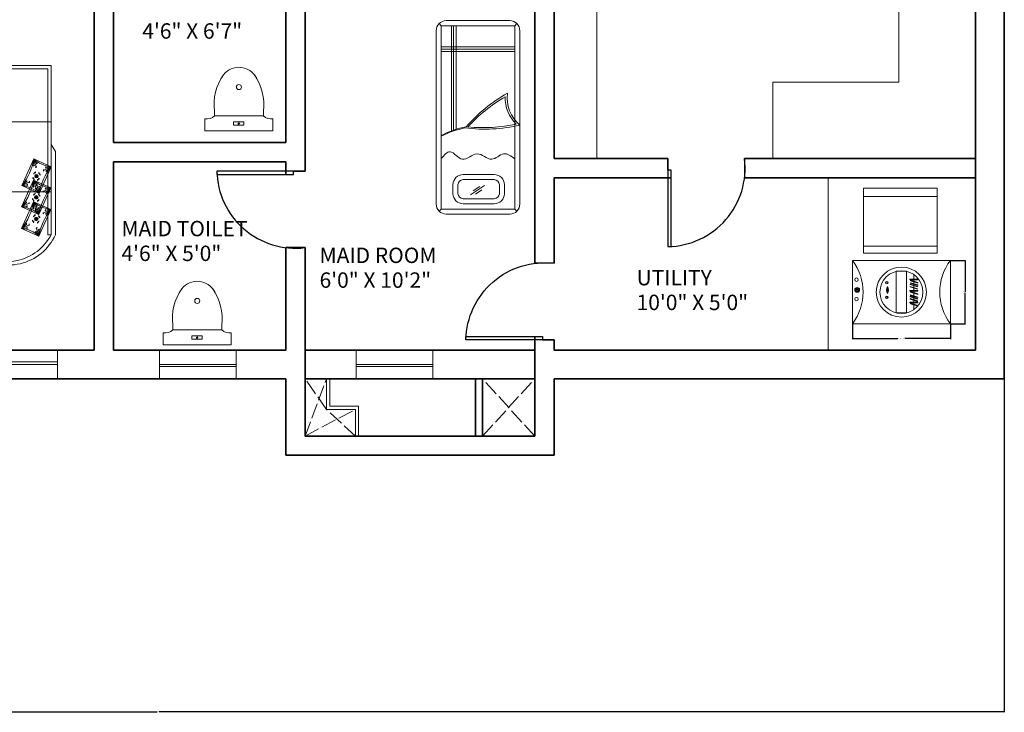
# Model space of a CAD drawing. Units: inches. Extents: x -61 to 1599, y -1316 to 257.
# Tile 167 of 204: x 1214 to 1523, y -1316 to -1099. Entities that reach past the tile are written whole.
import ezdxf

# ---------------------------------------------------------------- set-up
doc = ezdxf.new("R2010")
doc.units = ezdxf.units.IN
doc.header["$MEASUREMENT"] = 0
doc.linetypes.add('ACAD_ISO02W100', pattern=[15, 12, -3])
for name, color, linetype, lineweight in [('A-ANNO-DIMS', 2, 'Continuous', 18), ('A-AREA-IDEN', 1, 'Continuous', 18), ('A-EQPM', 9, 'Continuous', 18), ('A-FLOR-CASE', 8, 'Continuous', 18), ('A-FLOR-FIXT', 8, 'Continuous', 18), ('A-FLOR-OPEN-HIDN', 8, 'ACAD_ISO02W100', 13), ('A-WALL-JAMB', 4, 'ACAD_ISO02W100', 25), ('DOORS', 2, 'Continuous', 25), ('FURNITURE', 83, 'Continuous', 18), ('WALLS', 4, 'Continuous', 35), ('WINDOWS', 220, 'Continuous', 18)]:
    doc.layers.add(name, color=color, linetype=linetype, lineweight=lineweight)
doc.styles.get("Standard").update_dxf_attribs({"font": 'arial.ttf'})
doc.dimstyles.get("Standard").update_dxf_attribs({"dimtxt": 0.18, "dimasz": 0.18, "dimexe": 0.18, "dimexo": 0.0625, "dimgap": 0.09, "dimtad": 0, "dimtih": 1, "dimtoh": 1, "dimdec": 0, "dimzin": 0, "dimdsep": 46, "dimlunit": 3, "dimtxsty": 'Standard', "dimcen": 0.09, "dimadec": 0, "dimazin": 0, "dimtfac": 1, "dimtdec": 0, "dimtofl": 0, "dimtmove": 0, "dimatfit": 3, "dimfxl": 1, "dimtolj": 1, "dimtzin": 0, "dimarcsym": 0})

# ---------------------------------------------------------------- blocks, each defined once
blk = doc.blocks.new('DOOR-SWING-24')
blk.add_line((0, 0), (0, 3.6))
blk.add_lwpolyline([(0, 0), (0, -24), (1.05, -24), (1.05, 0)], close=True)
blk.add_arc((-0.44, 0.62), 24.62, 271.0259, 6.9559)
blk = doc.blocks.new('WIN-24IN')
for p, q in [((0, 4.5), (0, 9)), ((0, 9), (0, 0)), ((24, 9), (24, 0)), ((0, 5.19), (24, 5.19)), ((0, 4.5), (24, 4.5))]:
    blk.add_line(p, q)
blk = doc.blocks.new('WIN-36IN-2')
for p, q in [((0, 9), (0, 0)), ((36, 9), (36, 0)), ((0, 5.26), (36, 5.26)), ((0, 4.5), (36, 4.5)), ((0, 4.5), (36, 4.5))]:
    blk.add_line(p, q)
blk = doc.blocks.new('WC-FLOOR-MOUNT')
for p, q in [((3.02, 4.69), (3.02, 6.17)), ((18.31, 4.69), (18.31, 6.17)), ((0, 0), (0, 3.75)), ((3.02, 4.69), (18.31, 4.69)), ((21.33, 0), (21.33, 3.75)), ((0, 0), (21.33, 0))]:
    blk.add_line(p, q)
blk.add_lwpolyline([(12.24, 1.73), (8.96, 1.73), (8.96, 2.81), (12.24, 2.81)], close=True)
for centre, radius in [((10.67, 13.73), 0.792), ((10.6, 2.27), 0.208)]:
    blk.add_circle(centre, radius)
for centre, radius, start, end in [((10.67, 13.73), 6.18, 27.6844, 141.4697), ((19.05, 8.26), 16.17, 144.824, 187.4232), ((2.28, 8.26), 16.17, 352.5768, 35.176), ((0.56, 7.25), 3.55, 260.8586, 313.6993), ((20.77, 7.25), 3.55, 226.3007, 279.1414)]:
    blk.add_arc(centre, radius, start, end)
blk = doc.blocks.new('WASHING-MACHINE')
for p, q in [((19.24, 4.47), (19.22, 15.41)), ((0.98, 10.64), (0.75, 10.64)), ((0.96, 11.16), (1.13, 11)), ((1.12, 10.28), (0.96, 10.12)), ((1.49, 11.38), (1.49, 11.15)), ((1.49, 10.12), (1.49, 9.89)), ((2.02, 11.15), (1.86, 10.99)), ((1.86, 10.28), (2.02, 10.12)), ((2.23, 10.64), (2, 10.64)), ((11, 9.47), (11, 11.68))]:
    blk.add_line(p, q)
for points in [[(30.68, 0), (0, 0), (0, 19.87), (30.68, 19.87)], [(16.98, 3.42), (13.7, 3.42), (13.7, 16.45), (16.98, 16.45)], [(20.43, 13.78), (18.01, 13.78), (18.01, 13.95), (20.43, 13.95)], [(18.09, 12.45), (20.41, 11.74), (20.35, 11.57), (18.04, 12.29)], [(18.21, 13.64), (20.52, 12.92), (20.47, 12.76), (18.16, 13.47)], [(18.22, 12.89), (20.53, 12.18), (20.48, 12.01), (18.17, 12.73)], [(20.44, 10.23), (18.02, 10.23), (18.02, 10.4), (20.44, 10.4)], [(18.1, 11.71), (20.41, 10.99), (20.36, 10.83), (18.05, 11.54)], [(18.22, 10.09), (20.53, 9.38), (20.48, 9.21), (18.17, 9.92)], [(20.45, 6.56), (18.03, 6.56), (18.03, 6.73), (20.45, 6.73)], [(18.1, 8.63), (20.42, 7.91), (20.37, 7.75), (18.05, 8.46)], [(18.11, 7.88), (20.42, 7.17), (20.37, 7), (18.06, 7.72)], [(18.23, 9.07), (20.54, 8.36), (20.49, 8.19), (18.18, 8.91)], [(18.23, 6.42), (20.54, 5.7), (20.49, 5.54), (18.18, 6.25)]]:
    blk.add_lwpolyline(points, close=True)
for centre, radius in [((15.34, 9.94), 7.85), ((15.34, 9.94), 7.85), ((15.34, 9.94), 6.71), ((1.28, 13.83), 0.526), ((10.77, 12.86), 0.381), ((10.77, 12.86), 0.289), ((1.49, 10.64), 0.742), ((1.49, 10.64), 0.513), ((1.49, 10.64), 0.178), ((1.49, 10.64), 0.07), ((1.28, 7.75), 0.526), ((10.77, 8.29), 0.381), ((10.77, 8.29), 0.289)]:
    blk.add_circle(centre, radius)
for centre, radius, start, end in [((-13.12, 9.94), 16.46, 322.8671, 37.1329), ((43.8, 9.94), 16.46, 142.8671, 217.1329), ((12.8, 10.57), 2.11, 148.4251, 211.5749), ((9.2, 10.57), 2.11, 328.4251, 31.5749)]:
    blk.add_arc(centre, radius, start, end)
blk = doc.blocks.new('UTILITY-CABINET')
for p, q in [((0, 17.69), (23.01, 17.69)), ((0, 2.1), (23.01, 2.1))]:
    blk.add_line(p, q)
blk.add_lwpolyline([(23.01, 0), (0, 0), (0, 20.31), (23.01, 20.31)], close=True)
blk = doc.blocks.new('MASTER-BEDROOM-CONSOLE')
for p, q in [((0, 44.89), (23.59, 44.89)), ((23.59, 37.78), (23.59, 9.44)), ((23.59, 37.78), (24.94, 35.59)), ((24.94, 35.59), (24.94, 9.46)), ((18.16, 33.23), (18.88, 30.7)), ((18.16, 33.23), (19.13, 31.83)), ((18.16, 33.23), (18.18, 31.17)), ((18.2, 28.51), (18.44, 28.87)), ((18.44, 28.87), (18.68, 29.23)), ((19.01, 27.84), (18.62, 28.02)), ((19.01, 27.84), (18.71, 27.53)), ((19.01, 27.84), (18.83, 27.45)), ((19.01, 27.84), (18.89, 28.25)), ((19.18, 28.23), (19.01, 27.84)), ((19.31, 28.15), (19.01, 27.84)), ((19.4, 27.66), (19.01, 27.84)), ((19.13, 27.43), (19.01, 27.84)), ((19.96, 28.55), (19.84, 28.97)), ((20.09, 28.14), (19.96, 28.55)), ((23.59, 30.8), (21.23, 29.65)), ((23.59, 30.8), (21.89, 30.59)), ((23.59, 30.8), (22.04, 29.44)), ((14.43, 24.88), (15.98, 26.24)), ((14.43, 24.88), (16.79, 26.03)), ((14.43, 24.88), (16.12, 25.09)), ((18.06, 27.07), (17.94, 27.48)), ((18.18, 26.66), (18.06, 27.07)), ((18.08, 26.59), (18.8, 24.06)), ((18.08, 26.59), (19.06, 25.19)), ((18.08, 26.59), (18.1, 24.53)), ((19.85, 22.45), (19.14, 24.98)), ((19.38, 26.52), (19.62, 26.88)), ((19.62, 26.88), (19.86, 27.23)), ((0, 22.89), (23.59, 22.89)), ((18.12, 21.87), (18.36, 22.23)), ((18.36, 22.23), (18.6, 22.59)), ((18.93, 21.2), (18.81, 21.61)), ((19.85, 22.45), (18.88, 23.85)), ((19.11, 21.59), (18.93, 21.2)), ((19.89, 21.91), (19.76, 22.33)), ((19.85, 22.45), (19.84, 24.51)), ((20.01, 21.5), (19.89, 21.91)), ((23.51, 24.16), (21.15, 23.01)), ((23.51, 24.16), (21.82, 23.95)), ((23.51, 24.16), (21.96, 22.8)), ((14.35, 18.24), (15.9, 19.6)), ((14.35, 18.24), (16.71, 19.39)), ((17.98, 20.43), (17.86, 20.84)), ((18.11, 20.02), (17.98, 20.43)), ((18.08, 19.82), (18.8, 17.29)), ((18.08, 19.82), (19.06, 18.42)), ((18.08, 19.82), (18.1, 17.76)), ((18.93, 21.2), (18.54, 21.38)), ((18.93, 21.2), (18.63, 20.89)), ((18.93, 21.2), (18.75, 20.81)), ((19.23, 21.51), (18.93, 21.2)), ((19.32, 21.02), (18.93, 21.2)), ((19.05, 20.79), (18.93, 21.2)), ((19.3, 19.88), (19.54, 20.24)), ((19.54, 20.24), (19.78, 20.59)), ((14.35, 18.24), (16.04, 18.45)), ((18.12, 15.1), (18.36, 15.46)), ((18.36, 15.46), (18.6, 15.82)), ((19.78, 15.81), (18.8, 17.21)), ((19.78, 15.81), (19.06, 18.34)), ((19.78, 15.81), (19.76, 17.87)), ((19.89, 15.14), (19.76, 15.56)), ((23.51, 17.39), (21.15, 16.24)), ((23.51, 17.39), (21.82, 17.18)), ((23.51, 17.39), (21.96, 16.03)), ((14.35, 11.47), (15.9, 12.83)), ((14.35, 11.47), (16.71, 12.62)), ((17.98, 13.66), (17.86, 14.08)), ((18.11, 13.25), (17.98, 13.66)), ((18.93, 14.43), (18.54, 14.61)), ((18.93, 14.43), (18.63, 14.12)), ((18.93, 14.43), (18.75, 14.04)), ((18.93, 14.43), (18.81, 14.84)), ((19.11, 14.82), (18.93, 14.43)), ((19.23, 14.74), (18.93, 14.43)), ((19.32, 14.26), (18.93, 14.43)), ((19.05, 14.02), (18.93, 14.43)), ((19.3, 13.11), (19.54, 13.47)), ((19.54, 13.47), (19.78, 13.83)), ((20.01, 14.73), (19.89, 15.14)), ((14.35, 11.47), (16.04, 11.68)), ((19.78, 9.04), (18.8, 10.44)), ((19.78, 9.04), (19.06, 11.57)), ((19.78, 9.04), (19.76, 11.1)), ((22.59, 9.44), (23.59, 9.44)), ((1, 3.75), (0, 3.75))]:
    blk.add_line(p, q)
for points in [[(0, 3.75), (0, 62.52), (23.59, 62.52), (23.59, 9.44)], [(1, 3.75), (1, 61.52), (22.59, 61.52), (22.59, 9.44)]]:
    blk.add_lwpolyline(points)
for points in [[(14.43, 24.88), (18.16, 33.23), (23.59, 30.8), (19.85, 22.45)], [(14.35, 18.24), (18.08, 26.59), (23.51, 24.16), (19.78, 15.81)], [(14.35, 11.47), (18.08, 19.82), (23.51, 17.39), (19.78, 9.04)]]:
    blk.add_lwpolyline(points, close=True)
for centre, radius in [((19.01, 27.84), 0.567), ((19.01, 27.84), 0.567), ((19.01, 27.84), 0.43), ((18.93, 21.2), 0.567), ((18.93, 21.2), 0.567), ((18.93, 21.2), 0.43), ((18.93, 14.43), 0.567), ((18.93, 14.43), 0.567), ((18.93, 14.43), 0.43)]:
    blk.add_circle(centre, radius)
for centre, radius, start, end in [((0.46, 36.13), 17.94, 321.1446, 350.6879), ((18.22, 30.96), 0.209, 99.3213, 167.2974), ((17.97, 31.22), 0.214, 280.2125, 346.4062), ((24.49, 40.12), 9.36, 227.4013, 264.4312), ((18.14, 31.38), 0.214, 280.2125, 346.4062), ((18.39, 31.12), 0.209, 99.3213, 167.2974), ((18.84, 30.92), 0.214, 280.2125, 346.4062), ((19.08, 30.66), 0.209, 99.3213, 167.2974), ((19.17, 31.62), 0.209, 99.3213, 167.2974), ((18.92, 31.88), 0.214, 280.2125, 346.4062), ((19.1, 32.04), 0.214, 280.2125, 346.4062), ((19.34, 31.78), 0.209, 99.3213, 167.2974), ((18.91, 30.5), 0.209, 99.3213, 167.2974), ((18.67, 30.75), 0.214, 280.2125, 346.4062), ((37.56, 19.55), 17.94, 141.1446, 170.6879), ((21.4, 29.53), 0.214, 145.4264, 211.62), ((21.41, 29.77), 0.214, 145.4264, 211.62), ((21.05, 29.54), 0.209, 324.5352, 32.5112), ((21.06, 29.78), 0.209, 324.5352, 32.5112), ((22.08, 30.7), 0.214, 145.4264, 211.62), ((22.07, 30.47), 0.214, 145.4264, 211.62), ((21.72, 30.71), 0.209, 324.5352, 32.5112), ((21.72, 30.48), 0.209, 324.5352, 32.5112), ((22.21, 29.32), 0.214, 145.4264, 211.62), ((22.22, 29.56), 0.214, 145.4264, 211.62), ((21.86, 29.33), 0.209, 324.5352, 32.5112), ((21.87, 29.56), 0.209, 324.5352, 32.5112), ((0.38, 29.49), 17.94, 321.1446, 350.6879), ((13.52, 15.57), 9.36, 47.4013, 84.4312), ((16.15, 26.12), 0.209, 144.5352, 212.5112), ((16.15, 26.35), 0.209, 144.5352, 212.5112), ((15.8, 26.13), 0.214, 325.4264, 31.62), ((15.8, 26.36), 0.214, 325.4264, 31.62), ((16.29, 24.97), 0.209, 144.5352, 212.5112), ((16.3, 25.2), 0.209, 144.5352, 212.5112), ((15.95, 25.21), 0.214, 325.4264, 31.62), ((15.94, 24.98), 0.214, 325.4264, 31.62), ((16.96, 25.9), 0.209, 144.5352, 212.5112), ((16.96, 26.14), 0.209, 144.5352, 212.5112), ((16.61, 25.91), 0.214, 325.4264, 31.62), ((16.61, 26.15), 0.214, 325.4264, 31.62), ((24.42, 33.48), 9.36, 227.4013, 264.4312), ((18.06, 24.74), 0.214, 280.2125, 346.4062), ((18.31, 24.48), 0.209, 99.3213, 167.2974), ((19.09, 24.98), 0.209, 99.3213, 167.2974), ((18.85, 25.24), 0.214, 280.2125, 346.4062), ((19.18, 24.77), 0.214, 100.2125, 166.4062), ((18.93, 25.02), 0.209, 279.3213, 347.2974), ((19.02, 25.4), 0.214, 280.2125, 346.4062), ((19.26, 25.14), 0.209, 99.3213, 167.2974), ((19.1, 25.18), 0.209, 279.3213, 347.2974), ((19.35, 24.93), 0.214, 100.2125, 166.4062), ((19.8, 24.72), 0.209, 279.3213, 347.2974), ((20.04, 24.46), 0.214, 100.2125, 166.4062), ((18.14, 24.32), 0.209, 99.3213, 167.2974), ((17.89, 24.58), 0.214, 280.2125, 346.4062), ((18.83, 23.86), 0.209, 99.3213, 167.2974), ((18.59, 24.11), 0.214, 280.2125, 346.4062), ((18.92, 23.64), 0.214, 100.2125, 166.4062), ((18.68, 23.9), 0.209, 279.3213, 347.2974), ((18.76, 24.28), 0.214, 280.2125, 346.4062), ((19, 24.02), 0.209, 99.3213, 167.2974), ((18.85, 24.06), 0.209, 279.3213, 347.2974), ((19.09, 23.8), 0.214, 100.2125, 166.4062), ((19.87, 24.3), 0.214, 100.2125, 166.4062), ((19.63, 24.56), 0.209, 279.3213, 347.2974), ((37.48, 12.91), 17.94, 141.1446, 170.6879), ((21.33, 22.89), 0.214, 145.4264, 211.62), ((21.33, 23.13), 0.214, 145.4264, 211.62), ((20.97, 22.9), 0.209, 324.5352, 32.5112), ((20.98, 23.14), 0.209, 324.5352, 32.5112), ((22, 24.06), 0.214, 145.4264, 211.62), ((21.99, 23.83), 0.214, 145.4264, 211.62), ((21.64, 23.84), 0.209, 324.5352, 32.5112), ((21.65, 24.07), 0.209, 324.5352, 32.5112), ((22.14, 22.68), 0.214, 145.4264, 211.62), ((22.14, 22.92), 0.214, 145.4264, 211.62), ((21.78, 22.69), 0.209, 324.5352, 32.5112), ((21.79, 22.92), 0.209, 324.5352, 32.5112), ((0.38, 22.72), 17.94, 321.1446, 350.6879), ((16.07, 19.48), 0.209, 144.5352, 212.5112), ((16.08, 19.71), 0.209, 144.5352, 212.5112), ((15.72, 19.49), 0.214, 325.4264, 31.62), ((15.72, 19.72), 0.214, 325.4264, 31.62), ((16.22, 18.56), 0.209, 144.5352, 212.5112), ((15.87, 18.57), 0.214, 325.4264, 31.62), ((16.88, 19.26), 0.209, 144.5352, 212.5112), ((16.89, 19.5), 0.209, 144.5352, 212.5112), ((16.53, 19.27), 0.214, 325.4264, 31.62), ((16.53, 19.51), 0.214, 325.4264, 31.62), ((24.42, 26.71), 9.36, 227.4013, 264.4312), ((19.02, 18.63), 0.214, 280.2125, 346.4062), ((19.26, 18.37), 0.209, 99.3213, 167.2974), ((13.44, 8.93), 9.36, 47.4013, 84.4312), ((16.21, 18.33), 0.209, 144.5352, 212.5112), ((15.86, 18.34), 0.214, 325.4264, 31.62), ((18.14, 17.55), 0.209, 99.3213, 167.2974), ((17.89, 17.81), 0.214, 280.2125, 346.4062), ((18.06, 17.97), 0.214, 280.2125, 346.4062), ((18.31, 17.71), 0.209, 99.3213, 167.2974), ((18.83, 17.09), 0.209, 99.3213, 167.2974), ((18.59, 17.35), 0.214, 280.2125, 346.4062), ((18.84, 17), 0.214, 100.2125, 166.4062), ((18.6, 17.26), 0.209, 279.3213, 347.2974), ((18.76, 17.51), 0.214, 280.2125, 346.4062), ((19, 17.25), 0.209, 99.3213, 167.2974), ((18.77, 17.42), 0.209, 279.3213, 347.2974), ((19.01, 17.16), 0.214, 100.2125, 166.4062), ((19.09, 18.21), 0.209, 99.3213, 167.2974), ((18.85, 18.47), 0.214, 280.2125, 346.4062), ((19.1, 18.13), 0.214, 100.2125, 166.4062), ((18.85, 18.38), 0.209, 279.3213, 347.2974), ((19.03, 18.54), 0.209, 279.3213, 347.2974), ((19.27, 18.29), 0.214, 100.2125, 166.4062), ((19.79, 17.66), 0.214, 100.2125, 166.4062), ((19.55, 17.92), 0.209, 279.3213, 347.2974), ((19.72, 18.08), 0.209, 279.3213, 347.2974), ((19.97, 17.82), 0.214, 100.2125, 166.4062), ((37.48, 6.14), 17.94, 141.1446, 170.6879), ((21.33, 16.12), 0.214, 145.4264, 211.62), ((21.33, 16.36), 0.214, 145.4264, 211.62), ((20.97, 16.13), 0.209, 324.5352, 32.5112), ((20.98, 16.37), 0.209, 324.5352, 32.5112), ((22, 17.3), 0.214, 145.4264, 211.62), ((21.99, 17.06), 0.214, 145.4264, 211.62), ((21.64, 17.07), 0.209, 324.5352, 32.5112), ((21.65, 17.3), 0.209, 324.5352, 32.5112), ((22.14, 15.91), 0.214, 145.4264, 211.62), ((22.14, 16.15), 0.214, 145.4264, 211.62), ((21.78, 15.92), 0.209, 324.5352, 32.5112), ((21.79, 16.15), 0.209, 324.5352, 32.5112), ((16.07, 12.71), 0.209, 144.5352, 212.5112), ((16.08, 12.94), 0.209, 144.5352, 212.5112), ((15.72, 12.72), 0.214, 325.4264, 31.62), ((15.72, 12.95), 0.214, 325.4264, 31.62), ((16.88, 12.5), 0.209, 144.5352, 212.5112), ((16.89, 12.73), 0.209, 144.5352, 212.5112), ((16.53, 12.5), 0.214, 325.4264, 31.62), ((16.53, 12.74), 0.214, 325.4264, 31.62), ((10.31, 16.05), 16.05, 230.0449, 335.7344), ((9.45, 17.04), 16.05, 233.9382, 331.7264), ((13.44, 2.16), 9.36, 47.4013, 84.4312), ((16.21, 11.56), 0.209, 144.5352, 212.5112), ((16.22, 11.79), 0.209, 144.5352, 212.5112), ((15.87, 11.8), 0.214, 325.4264, 31.62), ((15.86, 11.57), 0.214, 325.4264, 31.62), ((18.84, 10.23), 0.214, 100.2125, 166.4062), ((18.6, 10.49), 0.209, 279.3213, 347.2974), ((18.77, 10.65), 0.209, 279.3213, 347.2974), ((19.01, 10.39), 0.214, 100.2125, 166.4062), ((19.1, 11.36), 0.214, 100.2125, 166.4062), ((18.85, 11.61), 0.209, 279.3213, 347.2974), ((19.03, 11.77), 0.209, 279.3213, 347.2974), ((19.27, 11.52), 0.214, 100.2125, 166.4062), ((19.79, 10.89), 0.214, 100.2125, 166.4062), ((19.55, 11.15), 0.209, 279.3213, 347.2974), ((19.72, 11.31), 0.209, 279.3213, 347.2974), ((19.97, 11.05), 0.214, 100.2125, 166.4062)]:
    blk.add_arc(centre, radius, start, end)
for points in [[(18.2, 28.51), (18.19, 28.6), (18.17, 28.79), (18.44, 28.88), (18.78, 28.9), (18.67, 29.16), (18.68, 29.23)], [(19.4, 27.66), (19.36, 27.75), (19.28, 27.92), (19, 27.85), (18.71, 27.68), (18.66, 27.96), (18.62, 28.02)], [(19.31, 28.15), (19.3, 28.05), (19.29, 27.87), (19.01, 27.83), (18.67, 27.88), (18.73, 27.6), (18.71, 27.53)], [(19.13, 27.43), (19.17, 27.51), (19.25, 27.69), (19.02, 27.85), (18.69, 27.97), (18.87, 28.18), (18.89, 28.25)], [(19.18, 28.23), (19.1, 28.19), (18.93, 28.11), (18.99, 27.83), (19.17, 27.54), (18.89, 27.49), (18.83, 27.45)], [(20.09, 28.14), (20.12, 28.23), (20.2, 28.4), (19.97, 28.57), (19.65, 28.68), (19.83, 28.9), (19.84, 28.97)], [(18.18, 26.66), (18.22, 26.75), (18.3, 26.92), (18.07, 27.09), (17.75, 27.2), (17.93, 27.41), (17.94, 27.48)], [(19.38, 26.52), (19.37, 26.61), (19.34, 26.8), (19.61, 26.89), (19.96, 26.9), (19.85, 27.16), (19.86, 27.23)], [(18.12, 21.87), (18.11, 21.96), (18.09, 22.15), (18.36, 22.24), (18.7, 22.26), (18.59, 22.52), (18.6, 22.59)], [(19.05, 20.79), (19.09, 20.87), (19.17, 21.05), (18.94, 21.21), (18.62, 21.33), (18.8, 21.54), (18.81, 21.61)], [(19.11, 21.59), (19.02, 21.55), (18.85, 21.47), (18.92, 21.19), (19.09, 20.9), (18.81, 20.85), (18.75, 20.81)], [(20.01, 21.5), (20.05, 21.59), (20.12, 21.76), (19.89, 21.93), (19.57, 22.04), (19.75, 22.26), (19.76, 22.33)], [(18.11, 20.02), (18.14, 20.11), (18.22, 20.28), (17.99, 20.45), (17.67, 20.56), (17.85, 20.77), (17.86, 20.84)], [(19.32, 21.02), (19.28, 21.11), (19.2, 21.28), (18.92, 21.21), (18.63, 21.04), (18.58, 21.32), (18.54, 21.38)], [(19.23, 21.51), (19.22, 21.41), (19.21, 21.23), (18.93, 21.19), (18.59, 21.24), (18.65, 20.96), (18.63, 20.89)], [(19.3, 19.88), (19.29, 19.97), (19.27, 20.16), (19.54, 20.25), (19.88, 20.26), (19.77, 20.52), (19.78, 20.59)], [(18.12, 15.1), (18.11, 15.19), (18.09, 15.38), (18.36, 15.47), (18.7, 15.49), (18.59, 15.75), (18.6, 15.82)], [(20.01, 14.73), (20.05, 14.82), (20.12, 14.99), (19.89, 15.16), (19.57, 15.27), (19.75, 15.49), (19.76, 15.56)], [(18.11, 13.25), (18.14, 13.34), (18.22, 13.51), (17.99, 13.68), (17.67, 13.79), (17.85, 14.01), (17.86, 14.08)], [(19.32, 14.26), (19.28, 14.34), (19.2, 14.51), (18.92, 14.44), (18.63, 14.27), (18.58, 14.55), (18.54, 14.61)], [(19.23, 14.74), (19.22, 14.64), (19.21, 14.46), (18.93, 14.42), (18.59, 14.47), (18.65, 14.19), (18.63, 14.12)], [(19.05, 14.02), (19.09, 14.1), (19.17, 14.28), (18.94, 14.44), (18.62, 14.56), (18.8, 14.77), (18.81, 14.84)], [(19.11, 14.82), (19.02, 14.78), (18.85, 14.7), (18.92, 14.43), (19.09, 14.13), (18.81, 14.08), (18.75, 14.04)], [(19.3, 13.11), (19.29, 13.2), (19.27, 13.39), (19.54, 13.48), (19.88, 13.49), (19.77, 13.75), (19.78, 13.83)]]:
    blk.add_open_spline(points, degree=3, knots=[0, 0, 0, 0, 0.249187, 0.498374, 0.766554, 1.034734, 1.034734, 1.034734, 1.034734])
blk = doc.blocks.new('*D672')
at = {"layer": 'A-ANNO-DIMS', "color": 0, "lineweight": -2, "transparency": 16777216}
for p, q in [((1475.13, -1194.01), (1475.13, -1198.73)), ((1505.81, -1194.01), (1505.81, -1198.73)), ((1475.31, -1198.55), (1489.35, -1198.55)), ((1505.63, -1198.55), (1491.59, -1198.55))]:
    blk.add_line(p, q, dxfattribs=at)
at = {"layer": 'A-ANNO-DIMS', "color": 0, "transparency": 16777216}
for points in [[(1475.31, -1198.52), (1475.31, -1198.58), (1475.13, -1198.55)], [(1505.63, -1198.52), (1505.63, -1198.58), (1505.81, -1198.55)]]:
    blk.add_solid(points, dxfattribs=at)
at = {"layer": 'DEFPOINTS', "color": 0, "transparency": 16777216}
for p in [(1475.13, -1193.95), (1505.81, -1193.95), (1505.81, -1198.55)]:
    blk.add_point(p, dxfattribs=at)
at = {"layer": 'A-ANNO-DIMS', "color": 0, "transparency": 16777216, "insert": (1490.47, -1198.55), "char_height": 0.18, "attachment_point": 5}
blk.add_mtext('\\A1;WASHER 31 TYP.', dxfattribs=at)
blk = doc.blocks.new('*D673')
at = {"layer": 'A-ANNO-DIMS', "color": 0, "lineweight": -2, "transparency": 16777216}
for p, q in [((1505.87, -1174.07), (1510.59, -1174.07)), ((1510.41, -1174.25), (1510.41, -1183.83)), ((1510.41, -1193.77), (1510.41, -1184.19)), ((1505.87, -1193.95), (1510.59, -1193.95))]:
    blk.add_line(p, q, dxfattribs=at)
at = {"layer": 'A-ANNO-DIMS', "color": 0, "transparency": 16777216}
for points in [[(1510.38, -1174.25), (1510.44, -1174.25), (1510.41, -1174.07)], [(1510.38, -1193.77), (1510.44, -1193.77), (1510.41, -1193.95)]]:
    blk.add_solid(points, dxfattribs=at)
at = {"layer": 'DEFPOINTS', "color": 0, "transparency": 16777216}
for p in [(1505.81, -1174.07), (1510.41, -1174.07), (1505.81, -1193.95)]:
    blk.add_point(p, dxfattribs=at)
at = {"layer": 'A-ANNO-DIMS', "color": 0, "transparency": 16777216, "insert": (1510.41, -1184.01), "char_height": 0.18, "attachment_point": 5}
blk.add_mtext('\\A1;20 TYP.', dxfattribs=at)
blk = doc.blocks.new('*D690')
at = {"layer": 'A-ANNO-DIMS', "color": 0, "lineweight": -2, "transparency": 16777216}
for p, q in [((992.7, -1211.23), (992.7, -1315.72)), ((1522.7, -1211.23), (1522.7, -1315.72)), ((992.88, -1315.54), (1257.41, -1315.54)), ((1522.52, -1315.54), (1257.99, -1315.54))]:
    blk.add_line(p, q, dxfattribs=at)
at = {"layer": 'A-ANNO-DIMS', "color": 0, "transparency": 16777216}
for points in [[(992.88, -1315.51), (992.88, -1315.57), (992.7, -1315.54)], [(1522.52, -1315.51), (1522.52, -1315.57), (1522.7, -1315.54)]]:
    blk.add_solid(points, dxfattribs=at)
at = {"layer": 'DEFPOINTS', "color": 0, "transparency": 16777216}
for p in [(992.7, -1211.17), (1522.7, -1211.17), (1522.7, -1315.54)]:
    blk.add_point(p, dxfattribs=at)
at = {"layer": 'A-ANNO-DIMS', "color": 0, "transparency": 16777216, "insert": (1257.7, -1315.54), "char_height": 0.18, "attachment_point": 5}
blk.add_mtext('\\A1;530', dxfattribs=at)

msp = doc.modelspace()

# ---------------------------------------------------------------- linework, layer by layer
at = {"layer": 'A-FLOR-CASE'}
for p, q in [((1489.7028, -1118.169), (1489.7028, -1029.169)), ((1395.0519, -1058.2566), (1395.0519, -1142.169)), ((1489.7028, -1118.169), (1450.2349, -1118.169)), ((1450.2349, -1118.169), (1450.2349, -1142.169)), ((1467.5747, -1202.169), (1467.5747, -1148.169))]:
    msp.add_line(p, q, dxfattribs=at)
at = {"layer": 'A-FLOR-OPEN-HIDN', "ltscale": 0.4}
for p, q in [((1303.7028, -1229.169), (1310.4306, -1211.169)), ((1310.4306, -1220.7676), (1303.7028, -1211.169)), ((1359.272, -1229.169), (1375.7028, -1211.169)), ((1375.7028, -1229.169), (1359.272, -1211.169)), ((1303.7028, -1229.169), (1319.4965, -1220.7676)), ((1319.4965, -1229.169), (1310.4306, -1220.7676))]:
    msp.add_line(p, q, dxfattribs=at)
at = {"layer": 'A-FLOR-OPEN-HIDN'}
for p, q in [((1310.4306, -1211.169), (1310.4306, -1220.7676)), ((1311.4306, -1211.169), (1311.4306, -1219.7676)), ((1310.4306, -1220.7676), (1319.4965, -1220.7676)), ((1311.4306, -1219.7676), (1320.4965, -1219.7676)), ((1319.4965, -1220.7676), (1319.4965, -1229.169)), ((1320.4965, -1219.7676), (1320.4965, -1229.169))]:
    msp.add_line(p, q, dxfattribs=at)
at = {"layer": 'A-WALL-JAMB'}
for p, q in [((1417.3522, -1142.169), (1417.3522, -1148.169)), ((1441.3522, -1142.169), (1441.3522, -1148.169)), ((1303.7028, -1146.0672), (1297.7028, -1146.0672)), ((1303.7028, -1170.0672), (1297.7028, -1170.0672)), ((1381.7028, -1174.9875), (1375.7028, -1174.9919)), ((1381.7028, -1198.9875), (1375.7028, -1198.9875))]:
    msp.add_line(p, q, dxfattribs=at)
at = {"layer": 'FURNITURE'}
for p, q in [((1346.3698, -1100.5135), (1345.7148, -1099.8585)), ((1349.5985, -1133.5005), (1349.5985, -1100.5135)), ((1350.1865, -1133.2891), (1350.1865, -1100.5135)), ((1351.0588, -1133.0003), (1351.0588, -1100.5135)), ((1369.4076, -1100.5135), (1370.0626, -1099.8585)), ((1369.4076, -1107.1545), (1346.3698, -1107.1545)), ((1369.4076, -1107.8638), (1346.3698, -1107.8638)), ((1369.4076, -1108.6332), (1346.3698, -1108.6332)), ((1359.8729, -1150.6342), (1355.5662, -1153.521)), ((1356.3763, -1152.2335), (1358.413, -1150.8765)), ((1357.072, -1153.2777), (1359.1087, -1151.9207)), ((1346.3698, -1157.9774), (1345.7148, -1158.6324)), ((1370.0626, -1158.6324), (1369.4076, -1157.9774))]:
    msp.add_line(p, q, dxfattribs=at)
for points in [[(1347.9511, -1098.9322), (1367.8263, -1098.9322, -0.41421356), (1370.989, -1102.0949), (1370.989, -1156.3961, -0.41421356), (1367.8263, -1159.5587), (1347.9511, -1159.5587, -0.41421356), (1344.7885, -1156.3961), (1344.7885, -1102.0949, -0.41421356)], [(1353.197, -1147.1816), (1362.9839, -1147.1816, -0.41421356), (1366.1465, -1150.3443), (1366.1465, -1153.1602, -0.41421356), (1362.9839, -1156.3228), (1353.197, -1156.3228, -0.41421356), (1350.0344, -1153.1602), (1350.0344, -1150.3443, -0.41421356)], [(1353.197, -1148.7629), (1362.9839, -1148.7629, -0.41421356), (1364.5652, -1150.3443), (1364.5652, -1153.1602, -0.41421356), (1362.9839, -1154.7415), (1353.197, -1154.7415, -0.41421356), (1351.6157, -1153.1602), (1351.6157, -1150.3443, -0.41421356)]]:
    msp.add_lwpolyline(points, format="xyb", close=True, dxfattribs=at)
msp.add_lwpolyline([(1346.3698, -1100.5135), (1369.4076, -1100.5135), (1369.4076, -1157.9774), (1346.3698, -1157.9774)], close=True, dxfattribs=at)
for centre, radius, start, end in [((1390.8702, -1164.0087), 48.5558, 119.302799, 139.065497), ((1378.0028, -1123.1891), 11.0029, 172.042189, 230.397858), ((1390.7906, -1164.772), 48.5558, 120.122754, 137.951503), ((1377.4118, -1123.3232), 11.0029, 177.136894, 226.788842), ((1359.4332, -1083.9234), 48.5558, 264.446321, 282.422187), ((1360.2263, -1162.1479), 30.5553, 101.397161, 116.967867), ((1359.9164, -1162.5088), 30.5553, 101.397161, 116.317614), ((1359.953, -1084.3818), 48.5558, 262.813151, 283.137248)]:
    msp.add_arc(centre, radius, start, end, dxfattribs=at)
msp.add_open_spline([(1369.4076, -1142.2411), (1368.2379, -1141.3554), (1365.818, -1139.5231), (1361.9669, -1143.9912), (1357.6119, -1138.7891), (1353.0321, -1144.3686), (1349.3585, -1138.5328), (1347.2784, -1141.0698), (1346.3698, -1142.1779)], degree=3, knots=[0, 0, 0, 0, 3.84254534, 7.94890144, 12.81558195, 17.74158221, 22.25649, 25.75782552, 25.75782552, 25.75782552, 25.75782552], dxfattribs=at)
at = {"layer": 'WALLS'}
for p, q in [((1522.7028, -1211.169), (1522.7028, -837.0151)), ((1513.7028, -1052.169), (1513.7028, -1148.169)), ((1237.7028, -1058.169), (1237.7028, -1202.169)), ((1243.7028, -1058.169), (1243.7028, -1137.169)), ((1297.7028, -1058.169), (1297.7028, -1137.169)), ((1381.7028, -1074.169), (1381.7028, -1142.169)), ((1303.7028, -1080.169), (1303.7028, -1146.0672)), ((1375.7028, -1080.169), (1375.7028, -1174.9919)), ((1243.7028, -1137.169), (1297.7028, -1137.169)), ((1243.7028, -1143.169), (1243.7028, -1202.169)), ((1243.7028, -1143.169), (1297.7028, -1143.169)), ((1297.7028, -1143.169), (1297.7028, -1147.1172)), ((1381.7028, -1142.169), (1417.3522, -1142.169)), ((1441.3522, -1142.169), (1513.7028, -1142.169)), ((1381.7028, -1148.169), (1381.7028, -1174.9875)), ((1381.7028, -1148.169), (1418.4022, -1148.169)), ((1441.3477, -1148.169), (1513.7028, -1148.169)), ((1513.7028, -1202.169), (1513.7028, -1148.169)), ((1297.7028, -1170.0628), (1297.7028, -1202.169)), ((1303.7028, -1170.0672), (1303.7028, -1211.169)), ((1375.7028, -1197.9375), (1375.7028, -1211.169)), ((1381.7028, -1198.9875), (1381.7028, -1202.169)), ((1065.7028, -1202.169), (1215.7028, -1202.169)), ((1215.7028, -1202.169), (1237.7028, -1202.169)), ((1243.7028, -1202.169), (1297.7028, -1202.169)), ((1303.7028, -1202.169), (1305.7028, -1202.169)), ((1305.7028, -1202.169), (1375.7028, -1202.169)), ((1381.7028, -1202.169), (1513.7028, -1202.169)), ((992.7028, -1211.169), (1215.7028, -1211.169)), ((1215.7028, -1211.169), (1297.7028, -1211.169)), ((1297.7028, -1211.169), (1297.7028, -1235.169)), ((1303.7028, -1211.169), (1305.7028, -1211.169)), ((1303.7028, -1211.169), (1303.7028, -1229.169)), ((1305.7028, -1211.169), (1375.7028, -1211.169)), ((1357.1436, -1229.169), (1357.1436, -1211.169)), ((1359.272, -1229.169), (1359.272, -1211.169)), ((1375.7028, -1211.169), (1375.7028, -1229.169)), ((1381.7028, -1211.169), (1522.7028, -1211.169)), ((1381.7028, -1211.169), (1381.7028, -1235.169)), ((1375.7028, -1229.169), (1303.7028, -1229.169)), ((1381.7028, -1235.169), (1297.7028, -1235.169))]:
    msp.add_line(p, q, dxfattribs=at)

# ---------------------------------------------------------------- block references
at = {"layer": 'A-EQPM'}
msp.add_blockref('WASHING-MACHINE', (1475.133, -1193.9451), dxfattribs=at)
at = {"layer": 'A-FLOR-CASE'}
msp.add_blockref('UTILITY-CABINET', (1478.634, -1171.7621), dxfattribs=at)
at = {"layer": 'A-FLOR-FIXT'}
for p in [(1272.349, -1133.4567), (1259.2982, -1200.5213)]:
    msp.add_blockref('WC-FLOOR-MOUNT', p, dxfattribs=at)
at = {"layer": 'DOORS'}
msp.add_blockref('DOOR-SWING-24', (1417.3522, -1145.769), dxfattribs=at)
at = {"layer": 'DOORS', "rotation": 270.0000000000005}
msp.add_blockref('DOOR-SWING-24', (1300.1028, -1146.0672), dxfattribs=at)
at = {"layer": 'DOORS', "extrusion": (0, 0, -1), "zscale": -1, "rotation": 90.00000000000048}
msp.add_blockref('DOOR-SWING-24', (-1378.1028, -1198.9875), dxfattribs=at)
at = {"layer": 'FURNITURE'}
msp.add_blockref('MASTER-BEDROOM-CONSOLE', (1200.602, -1175.5131), dxfattribs=at)
at = {"layer": 'WINDOWS'}
msp.add_blockref('WIN-36IN-2', (1190.158, -1211.1691), dxfattribs=at)
at = {"layer": 'WINDOWS', "rotation": 180}
for p in [(1282.1139, -1202.1689), (1343.7033, -1202.1689)]:
    msp.add_blockref('WIN-24IN', p, dxfattribs=at)

# ---------------------------------------------------------------- texts
at = {"layer": 'A-AREA-IDEN'}
for s, height, p in [('4\'6" X 6\'7"', 4.832098, (1252.7407, -1104.5856)), ('MAID TOILET', 4.832098, (1246.2172, -1166.5142)), ('4\'6" X 5\'0"', 4.832098, (1246.2172, -1174.2766)), ('MAID ROOM', 4.8321, (1308.2598, -1174.9019)), ('6\'0" X 10\'2"', 4.832098, (1308.2598, -1182.6643)), ('UTILITY', 4.8321, (1407.5332, -1181.8915)), ('10\'0" X 5\'0"', 4.832098, (1407.5332, -1189.6539))]:
    msp.add_text(s, height=height, dxfattribs=at).set_placement(p)

# ---------------------------------------------------------------- dimensions: what is measured, and where the dimension line sits
at = {"layer": 'A-ANNO-DIMS'}
dim = msp.add_linear_dim(base=(1510.4117, -1174.0743), p1=(1505.8101, -1193.9451), p2=(1505.8101, -1174.0743), angle=90, text='<> TYP.', dimstyle='Standard', override={"dimdec": 0, "dimlfac": 1, "dimrnd": 0, "dimzin": 0, "dimdsep": 46, "dimlunit": 2}, dxfattribs=at)
dim.commit()
dim.dimension.update_dxf_attribs({"geometry": '*D673', "text_midpoint": (1510.4117, -1184.0097)})
dim = msp.add_linear_dim(base=(1505.8101, -1198.5467), p1=(1475.1329, -1193.9451), p2=(1505.8101, -1193.9451), text='WASHER <> TYP.', dimstyle='Standard', override={"dimdec": 0, "dimlfac": 1, "dimrnd": 0, "dimzin": 0, "dimdsep": 46, "dimlunit": 2}, dxfattribs=at)
dim.commit()
dim.dimension.update_dxf_attribs({"geometry": '*D672', "text_midpoint": (1490.4715, -1198.5467)})
dim = msp.add_linear_dim(base=(1522.7028, -1315.5446), p1=(992.7028, -1211.169), p2=(1522.7028, -1211.169), dimstyle='Standard', override={"dimdec": 0, "dimlfac": 1, "dimrnd": 0, "dimzin": 0, "dimdsep": 46, "dimlunit": 2}, dxfattribs=at)
dim.commit()
dim.dimension.update_dxf_attribs({"geometry": '*D690', "text_midpoint": (1257.7028, -1315.5446)})

doc.saveas('drawing.dxf')
